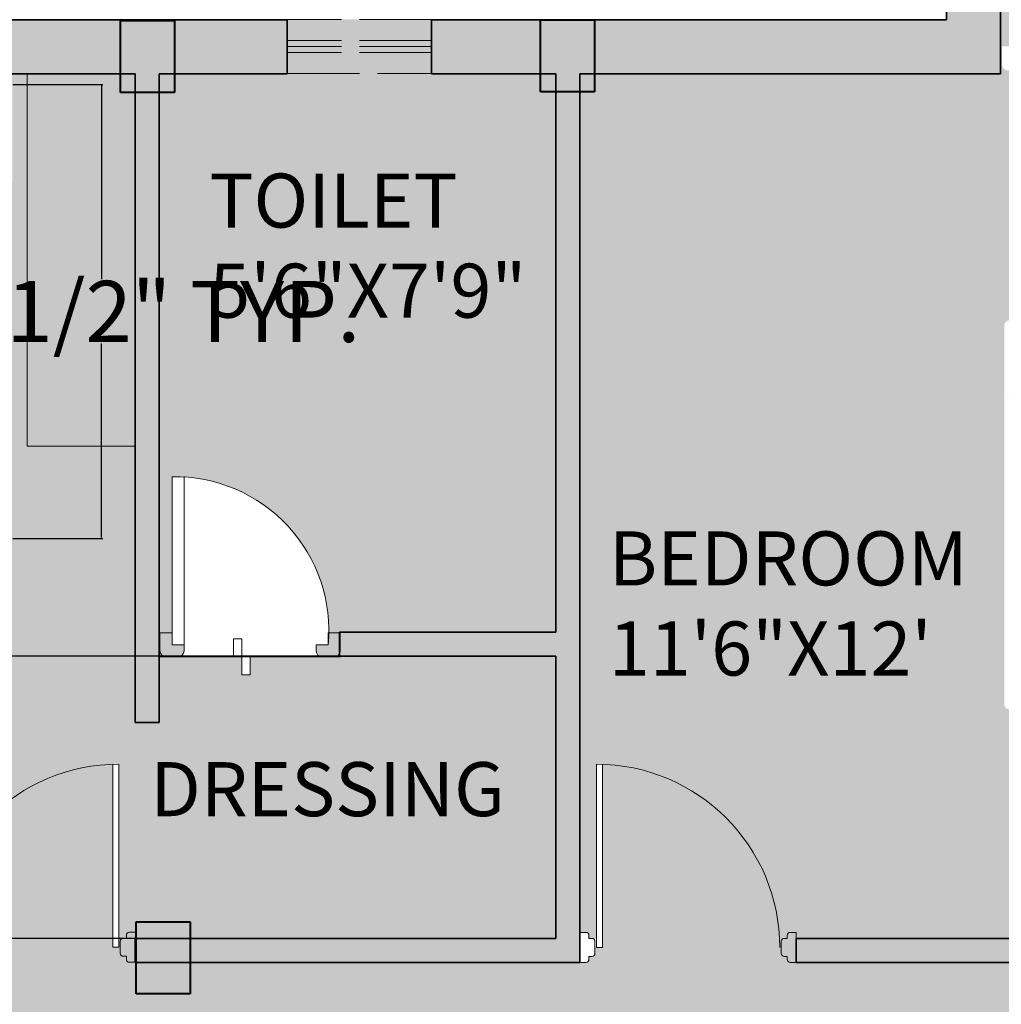
# Model space of a CAD drawing. Units: inches. Extents: x 1077 to 2505, y 1892 to 2728.
# Tile 15 of 26: x 1306 to 1470, y 2422 to 2586. Entities that reach past the tile are written whole.
import ezdxf

# ---------------------------------------------------------------- set-up
doc = ezdxf.new("R2010")
doc.units = ezdxf.units.IN
doc.linetypes.add('ACAD_ISO02W100', pattern=[15, 12, -3])
doc.layers.get('Defpoints').update_dxf_attribs({"color": 220, "linetype": 'ACAD_ISO02W100'})
for name, color, linetype, lineweight in [('00 FURNITURE', 15, 'Continuous', 15), ('A-ANNO-DIMS', 2, 'Continuous', 18), ('A-AREA-IDEN', 7, 'Continuous', 18), ('A-COLS', 7, 'Continuous', 40), ('A-DOOR', 4, 'Continuous', 18), ('A-FLOR-CASE', 8, 'Continuous', 18), ('A-GLAZ-VENT', 6, 'ACAD_ISO02W100', 13), ('A-WALL-PATT', 7, 'Continuous', 9), ('A_FUR 1', 5, 'Continuous', 5), ('WALL', 7, 'Continuous', 35)]:
    doc.layers.add(name, color=color, linetype=linetype, lineweight=lineweight)
doc.layers.add('A-FLOR-CASE-PATT', color=32, linetype='Continuous', lineweight=9, true_color=0xcd6928)
doc.layers.add('A-FLOR-PATT', color=254, linetype='Continuous', lineweight=9, true_color=0xd7ebd2)
doc.styles.get("Standard").update_dxf_attribs({"font": 'arial.ttf'})
doc.dimstyles.get("Standard").update_dxf_attribs({"dimtxt": 10.18, "dimasz": 0.18, "dimexe": 0.18, "dimexo": 0.0625, "dimgap": 0.09, "dimtad": 0, "dimtih": 1, "dimtoh": 1, "dimdec": 0, "dimzin": 0, "dimdsep": 46, "dimlunit": 3, "dimtxsty": 'Standard', "dimcen": 0.09, "dimadec": 0, "dimazin": 0, "dimtfac": 1, "dimtdec": 0, "dimtofl": 0, "dimtmove": 0, "dimatfit": 3, "dimfxl": 1, "dimtolj": 1, "dimtzin": 0, "dimarcsym": 0})

# ---------------------------------------------------------------- blocks, each defined once
blk = doc.blocks.new('DDD')
at = {"layer": '00 FURNITURE'}
for p, q in [((-12579.77, -15859.53), (-12579.77, -15829.05)), ((-12578.77, -15859.53), (-12578.77, -15829.03)), ((-12612.02, -15857.03), (-12612.02, -15862.03)), ((-12611.02, -15857.03), (-12612.02, -15857.03)), ((-12610.52, -15858.03), (-12610.52, -15857.53)), ((-12577.52, -15858.03), (-12577.52, -15857.53)), ((-12577.02, -15857.03), (-12576.02, -15857.03)), ((-12576.02, -15857.03), (-12576.02, -15862.03)), ((-12578.77, -15859.53), (-12579.77, -15859.53)), ((-12610.52, -15861.53), (-12610.52, -15861.03)), ((-12577.52, -15861.53), (-12577.52, -15861.03)), ((-12612.02, -15862.03), (-12611.02, -15862.03)), ((-12576.02, -15862.03), (-12577.02, -15862.03))]:
    blk.add_line(p, q, dxfattribs=at)
for points in [[(-12610.52, -15861.03), (-12610.02, -15861.03, 0.414214), (-12609.52, -15860.53), (-12609.52, -15858.53, 0.414214), (-12610.02, -15858.03), (-12610.52, -15858.03)], [(-12577.52, -15861.03), (-12578.02, -15861.03, -0.414214), (-12578.52, -15860.53), (-12578.52, -15858.53, -0.414214), (-12578.02, -15858.03), (-12577.52, -15858.03)]]:
    blk.add_lwpolyline(points, format="xyb", dxfattribs=at)
for centre, radius, start, end in [((-12578.77, -15859.53), 30.5, 90, 180), ((-12611.02, -15857.53), 0.5, 0, 90), ((-12577.02, -15857.53), 0.5, 90, 180), ((-12611.02, -15861.53), 0.5, 270, 0), ((-12577.02, -15861.53), 0.5, 180, 270)]:
    blk.add_arc(centre, radius, start, end, dxfattribs=at)
blk = doc.blocks.new('ESTSET')
at = {"layer": 'A_FUR 1'}
for p, q in [((-10.44, 4.1), (-10.44, 32.1)), ((-8.44, 4.1), (-8.44, 32.1)), ((-36.44, 6.1), (-36.44, 3.1)), ((-34.44, 6.1), (-36.44, 6.1)), ((-34.44, 4.1), (-34.44, 6.1)), ((-34.44, 4.1), (-34.44, 6.1)), ((-8.44, 4.1), (-8.44, 6.1)), ((-8.44, 6.1), (-6.44, 6.1)), ((-8.44, 4.1), (-8.44, 6.1)), ((-6.44, 6.1), (-6.44, 3.1)), ((-32.44, 4.1), (-34.44, 4.1)), ((-32.44, 4.1), (-34.44, 4.1)), ((-32.44, 3.1), (-32.44, 4.1)), ((-10.44, 3.1), (-10.44, 4.1)), ((-10.44, 4.1), (-8.44, 4.1)), ((-10.44, 4.1), (-8.44, 4.1)), ((-6.44, 2.1), (-36.44, 2.1)), ((-35.44, 2.1), (-33.44, 2.1)), ((-7.44, 2.1), (-9.44, 2.1))]:
    blk.add_line(p, q, dxfattribs=at)
for points in [[(-21.44, 2.1), (-18.67, 2.1), (-18.67, 5.1), (-20.06, 5.1)], [(-20.06, 5.1), (-20.06, -0.91)], [(-21.44, 2.1), (-21.44, -0.91), (-20.06, -0.91)]]:
    blk.add_lwpolyline(points, dxfattribs=at)
for centre, radius, start, end in [((-8.91, 6.46), 25.64, 88.9606, 185.2816), ((-35.44, 3.1), 1, 180, 270), ((-33.44, 3.1), 1, 270, 0), ((-9.44, 3.1), 1, 180, 270), ((-7.44, 3.1), 1, 270, 0)]:
    blk.add_arc(centre, radius, start, end, dxfattribs=at)
blk = doc.blocks.new('C1')
h = blk.add_hatch(color=256)
h.dxf.hatch_style = 1
h.paths.add_polyline_path([(1668.56, 2445.41), (1677.56, 2445.41), (1677.56, 2457.41), (1668.56, 2457.41)])
for p, q in [((1668.56, 2457.41), (1677.56, 2457.41)), ((1668.56, 2445.41), (1668.56, 2457.41)), ((1677.56, 2457.41), (1677.56, 2445.41)), ((1677.56, 2445.41), (1668.56, 2445.41))]:
    blk.add_line(p, q)
blk = doc.blocks.new('VENT-24')
for p, q in [((3.5, 24), (3.5, 0)), ((4.5, 24), (4.5, 0)), ((5.5, 24), (5.5, 0))]:
    blk.add_line(p, q)
blk.add_lwpolyline([(0, 0), (9, 0), (9, 24), (0, 24)], close=True)
blk = doc.blocks.new('*D33')
at = {"layer": 'A-ANNO-DIMS', "color": 0, "lineweight": -2, "transparency": 16777216}
for p, q in [((1305.15, 2575.38), (1320.12, 2575.38)), ((1319.94, 2575.2), (1319.94, 2542.94)), ((1319.94, 2499.96), (1319.94, 2532.23)), ((1305.15, 2499.78), (1320.12, 2499.78))]:
    blk.add_line(p, q, dxfattribs=at)
at = {"layer": 'A-ANNO-DIMS', "color": 0, "transparency": 16777216}
for points in [[(1319.91, 2575.2), (1319.97, 2575.2), (1319.94, 2575.38)], [(1319.91, 2499.96), (1319.97, 2499.96), (1319.94, 2499.78)]]:
    blk.add_solid(points, dxfattribs=at)
at = {"layer": 'Defpoints', "color": 0, "transparency": 16777216}
for p in [(1305.09, 2575.38), (1319.94, 2575.38), (1305.09, 2499.78)]:
    blk.add_point(p, dxfattribs=at)
at = {"layer": 'A-ANNO-DIMS', "color": 0, "transparency": 16777216, "insert": (1319.94, 2537.58), "char_height": 10.18, "attachment_point": 5}
blk.add_mtext('\\A1;6\'-3 1/2" TYP.', dxfattribs=at)
blk = doc.blocks.new('*D64')
at = {"layer": 'A-ANNO-DIMS', "color": 0, "lineweight": -2, "transparency": 16777216}
for p, q in [((1395.47, 2480.16), (1149.43, 2480.16)), ((1149.61, 2479.98), (1149.61, 2461.95)), ((1149.61, 2433.34), (1149.61, 2451.37)), ((1395.47, 2433.16), (1149.43, 2433.16))]:
    blk.add_line(p, q, dxfattribs=at)
at = {"layer": 'A-ANNO-DIMS', "color": 0, "transparency": 16777216}
for points in [[(1149.58, 2479.98), (1149.64, 2479.98), (1149.61, 2480.16)], [(1149.58, 2433.34), (1149.64, 2433.34), (1149.61, 2433.16)]]:
    blk.add_solid(points, dxfattribs=at)
at = {"layer": 'Defpoints', "color": 0, "transparency": 16777216}
for p in [(1149.61, 2480.16), (1395.53, 2480.16), (1395.53, 2433.16)]:
    blk.add_point(p, dxfattribs=at)
at = {"layer": 'A-ANNO-DIMS', "color": 0, "transparency": 16777216, "insert": (1149.61, 2456.66), "char_height": 10.18, "attachment_point": 5}
blk.add_mtext('\\A1;3\'-11"', dxfattribs=at)

msp = doc.modelspace()

# ---------------------------------------------------------------- hatches: boundary and pattern name
at = {"layer": 'A-FLOR-CASE-PATT', "transparency": 33554610}
h = msp.add_hatch(color=256, dxfattribs=at)
h.dxf.hatch_style = 1
h.paths.add_polyline_path([(1325.53, 2577.15), (1307.53, 2577.15), (1307.53, 2515.13), (1325.53, 2515.13)])
h.paths.add_polyline_path([(1476.35, 2451.18), (1476.35, 2433.16), (1547.53, 2433.16), (1547.53, 2437.11), (1547.53, 2451.18)])
at = {"layer": 'A-FLOR-PATT', "transparency": 33554559}
h = msp.add_hatch(color=256, dxfattribs=at)
h.dxf.hatch_style = 1
h.paths.add_polyline_path([(1395.53, 2577.16), (1374.83, 2577.16), (1350.83, 2577.19), (1350.83, 2577.16), (1329.53, 2577.16), (1329.53, 2480.16), (1329.53, 2469.16), (1325.53, 2469.16), (1325.53, 2515.13), (1307.53, 2515.13), (1307.53, 2577.16), (1269.31, 2577.16), (1221.31, 2577.15), (1221.31, 2577.16), (1187.53, 2577.16), (1187.53, 2433.16), (1289.53, 2433.16), (1289.53, 2429.16), (1263.53, 2429.16), (1187.53, 2429.16), (1187.53, 2395.02), (1187.53, 2395.02), (1187.53, 2371.02), (1187.53, 2371.02), (1187.53, 2307.16), (1259.53, 2307.16), (1259.53, 2399.16), (1263.53, 2399.16), (1263.53, 2307.16), (1289.53, 2307.16), (1289.53, 2306.23), (1325.53, 2306.23), (1325.53, 2307.16), (1329.53, 2307.16), (1329.53, 2306.23), (1365.53, 2306.23), (1365.53, 2307.16), (1432.53, 2307.16), (1432.53, 2088.16), (1547.53, 2088.16), (1547.53, 2140.08), (1511.53, 2140.08), (1511.53, 2267.16), (1475.53, 2267.16), (1475.53, 2303.16), (1468.53, 2303.16), (1468.53, 2307.16), (1547.53, 2307.16), (1547.53, 2348.22), (1547.53, 2396.22), (1547.53, 2429.16), (1435.53, 2429.16), (1435.53, 2433.16), (1476.35, 2433.16), (1476.35, 2451.18), (1547.53, 2451.18), (1547.53, 2577.16), (1499.53, 2577.16), (1499.53, 2586.16), (1547.53, 2586.16), (1547.53, 2642.16), (1518.18, 2642.16), (1518.18, 2642.05), (1494.15, 2642.05), (1494.15, 2642.16), (1469.53, 2642.16), (1469.53, 2577.16), (1399.53, 2577.16), (1399.53, 2429.16), (1325.53, 2429.16), (1325.53, 2433.16), (1329.53, 2433.16), (1395.53, 2433.16), (1395.53, 2480.16), (1359.53, 2480.16), (1359.53, 2484.16), (1395.53, 2484.16)])
h.paths.add_polyline_path([(1357.65, 2482.07), (1355.65, 2482.07), (1355.65, 2481.07, 0.414214), (1356.65, 2480.07), (1344.65, 2480.07), (1344.65, 2477.06), (1343.27, 2477.06), (1343.27, 2480.07), (1330.65, 2480.07, -0.414214), (1329.65, 2481.07), (1329.65, 2484.07), (1331.65, 2484.07), (1331.65, 2510.07, -0.446908)], flags=16)
h.paths.add_polyline_path([(1305.09, 2559.18), (1288.89, 2559.18), (1288.89, 2575.38), (1305.09, 2575.38)], flags=16)
h.paths.add_polyline_path([(1304.19, 2560.08), (1289.79, 2560.08), (1289.79, 2574.48), (1304.19, 2574.48)], flags=0)
h.paths.add_polyline_path([(1287.99, 2500.68, -0.414214), (1287.09, 2499.78), (1265.14, 2499.78), (1224.09, 2499.78, -0.414214), (1223.19, 2500.68), (1223.19, 2557.16), (1223.19, 2571.74), (1223.19, 2575.38), (1287.99, 2575.38), (1287.99, 2571.74), (1287.09, 2571.74, -0.414214), (1287.99, 2570.84)], flags=16)
h.paths.add_polyline_path([(1292.98, 2569.05, -1), (1300.92, 2569.05, -1)], flags=0)
h.paths.add_polyline_path([(1293.32, 2569.05, -1), (1300.58, 2569.05, -1)], flags=0)
h.paths.add_polyline_path([(1322.8, 2462.21), (1322.8, 2431.71), (1323.05, 2430.71), (1323.05, 2431.71), (1321.8, 2431.71), (1321.8, 2462.19, 0.404641), (1292.3, 2431.71), (1292.05, 2430.71, -0.414214), (1291.55, 2430.21), (1291.05, 2430.21), (1291.05, 2429.71, -0.414214), (1290.55, 2429.21), (1289.55, 2429.21), (1289.55, 2434.21), (1290.55, 2434.21, -0.414214), (1291.05, 2433.71), (1291.05, 2433.21), (1291.55, 2433.21, -0.414214), (1292.05, 2432.71), (1292.3, 2431.71, -0.414214)], flags=16)
h.paths.add_polyline_path([(1287.82, 2548.28, 0.292232), (1279.17, 2536.8, 0.052719), (1223.93, 2548.28), (1223.28, 2548.28), (1223.28, 2557.16), (1223.93, 2557.16), (1245.42, 2557.16, -0.117785), (1245.77, 2557.93, -0.059418), (1254.87, 2567.02, -0.379859), (1257.28, 2566.88, -0.02509), (1261.41, 2563.32, -0.025935), (1265.65, 2567.02, -0.379859), (1268.06, 2566.88, -0.061767), (1277.52, 2557.43, -0.069393), (1277.82, 2557.16), (1287.82, 2557.16)], flags=0)
h.paths.add_polyline_path([(1263.47, 2548.28), (1260.56, 2548.28, -0.015371), (1258.01, 2546.13, -0.429576), (1255.37, 2546.06, -0.016036), (1252.69, 2548.28), (1223.28, 2548.28), (1223.28, 2554.42), (1246.78, 2554.42, 0.055344), (1255.37, 2546.06, 0.331768), (1257.52, 2545.74, 0.027343), (1262, 2549.64, 0.00919)], flags=0)
h.paths.add_polyline_path([(1295.56, 2568.34), (1296.87, 2569.09), (1296.87, 2570.6, 0.399698), (1295.39, 2569.05, 0.119004)], flags=0)
h.paths.add_polyline_path([(1295.21, 2569.05, -1), (1298.68, 2569.05, -1)], flags=0)
h.paths.add_polyline_path([(1296.95, 2568.96), (1297.03, 2569), (1297.03, 2569.09), (1296.99, 2569.11), (1296.91, 2568.98)], flags=0)
h.paths.add_polyline_path([(1402.28, 2462.19, -0.414214), (1432.78, 2431.69), (1433.03, 2432.69), (1432.78, 2431.69, 0.404641), (1403.28, 2462.17), (1403.28, 2431.69), (1402.03, 2431.69), (1402.03, 2430.69, -0.414214), (1401.53, 2430.19), (1401.03, 2430.19), (1401.03, 2429.69, -0.414214), (1400.53, 2429.19), (1399.53, 2429.19), (1399.53, 2434.19), (1400.53, 2434.19, -0.414214), (1401.03, 2433.69), (1401.03, 2433.19), (1401.53, 2433.19, -0.414214), (1402.03, 2432.69)], flags=16)
h.paths.add_polyline_path([(1470.16, 2535.21, -0.414214), (1471.06, 2536.11), (1527.54, 2536.11), (1542.12, 2536.11), (1545.76, 2536.11), (1545.76, 2471.31), (1542.12, 2471.31), (1542.12, 2472.21, -0.414214), (1541.22, 2471.31), (1471.06, 2471.31, -0.414214), (1470.16, 2472.21), (1470.16, 2494.16)], flags=16)
h.paths.add_polyline_path([(1483.07, 2536.11, 0.253465), (1480.11, 2526.15, 0.2538), (1470.15, 2523.19)], flags=16)
h.paths.add_polyline_path([(1223.19, 2512.69, 0.253465), (1233.14, 2509.74, 0.2538), (1236.1, 2499.77)], flags=16)
h.paths.add_polyline_path([(1469.77, 2578.72), (1469.77, 2581.72), (1471.77, 2581.72), (1471.77, 2607.72, -0.01951), (1473.77, 2607.68), (1473.77, 2579.72), (1473.77, 2578.72, -0.414214), (1472.77, 2577.72), (1470.77, 2577.72, -0.414214)], flags=16)
h.paths.add_polyline_path([(1382.46, 2398.13), (1395.04, 2398.13), (1395.04, 2399.74), (1382.46, 2399.74)], flags=16)
h.paths.add_polyline_path([(1379.94, 2397.18), (1379.94, 2389.82), (1380.5, 2389.82), (1380.5, 2396.05, -0.41429), (1381.06, 2396.61), (1396.47, 2396.61, -0.414213), (1397.03, 2396.05), (1397.03, 2389.82), (1397.59, 2389.82), (1397.59, 2397.18)], flags=16)
h.paths.add_polyline_path([(1263.37, 2428.14), (1263.37, 2426.14, -0.414214), (1262.37, 2425.14), (1261.37, 2425.14), (1233.41, 2425.14, 0.400854), (1259.37, 2401.04), (1259.37, 2401.14), (1261.37, 2401.14, -0.446908), (1233.37, 2427.14), (1259.37, 2427.14), (1259.37, 2429.14), (1262.37, 2429.14, -0.414214)], flags=16)
h.paths.add_polyline_path([(1404.79, 2398.13), (1417.37, 2398.13), (1417.37, 2399.74), (1404.79, 2399.74)], flags=16)
h.paths.add_polyline_path([(1402.27, 2397.18), (1404.79, 2398.13), (1417.37, 2398.13), (1419.92, 2397.18)], flags=16)
h.paths.add_polyline_path([(1432.26, 2383.16), (1432.26, 2370.59), (1433.87, 2370.59), (1433.87, 2383.16)], flags=16)
h.paths.add_polyline_path([(1431.3, 2385.69), (1423.84, 2385.69), (1423.84, 2385.13), (1430.18, 2385.13, -0.41429), (1430.74, 2384.57), (1430.74, 2369.16, -0.414237), (1430.18, 2368.6), (1423.84, 2368.6), (1423.84, 2368.03), (1431.3, 2368.03)], flags=16)
h.paths.add_polyline_path([(1417.37, 2351.16), (1417.37, 2349.54), (1418.9, 2349.54, 0.414236), (1419.92, 2350.56), (1419.92, 2352.11)], flags=16)
h.paths.add_polyline_path([(1395.04, 2351.16), (1395.04, 2349.54), (1396.58, 2349.54, 0.414235), (1397.59, 2350.56), (1397.59, 2352.11)], flags=16)
h.paths.add_polyline_path([(1366.7, 2370.05), (1365.09, 2370.05), (1365.09, 2368.52, 0.414235), (1366.11, 2367.5), (1367.66, 2367.5)], flags=16)
h.paths.add_polyline_path([(1419.36, 2359.47), (1419.36, 2353.24, -0.41419), (1418.8, 2352.68), (1403.39, 2352.68, -0.414137), (1402.83, 2353.24), (1402.83, 2359.47), (1397.03, 2359.47), (1397.03, 2353.24, -0.414189), (1396.47, 2352.68), (1381.06, 2352.68, -0.414137), (1380.5, 2353.24), (1380.5, 2359.47)], flags=16)
h.paths.add_polyline_path([(1222.29, 2559.18), (1206.09, 2559.18), (1206.09, 2575.38), (1222.29, 2575.38)], flags=16)
h.paths.add_polyline_path([(1221.39, 2560.08), (1206.99, 2560.08), (1206.99, 2574.48), (1221.39, 2574.48)], flags=0)
h.paths.add_polyline_path([(1482, 2577.72), (1482, 2580.73), (1483.38, 2580.73), (1483.38, 2577.72), (1484.77, 2577.72), (1484.77, 2574.72), (1483.38, 2574.72), (1483.38, 2577.72)], flags=16)
h.paths.add_polyline_path([(1266.37, 2415.53), (1266.37, 2414.14), (1263.37, 2414.14), (1263.37, 2415.53), (1260.36, 2415.53), (1260.36, 2416.91), (1263.37, 2416.91), (1263.37, 2415.53)], flags=16)
h.paths.add_polyline_path([(1210.26, 2569.05, -1), (1218.19, 2569.05, -1)], flags=0)
h.paths.add_polyline_path([(1210.6, 2569.05, -1), (1217.85, 2569.05, -1)], flags=0)
h.paths.add_polyline_path([(1212.84, 2568.34), (1214.15, 2569.09), (1214.15, 2570.6, 0.399698), (1212.67, 2569.05, 0.119004)], flags=0)
h.paths.add_polyline_path([(1212.49, 2569.05, -1), (1215.96, 2569.05, -1)], flags=0)
h.paths.add_polyline_path([(1214.23, 2568.96), (1214.3, 2568.91), (1214.3, 2569)], flags=0)
h.paths.add_polyline_path([(1507.18, 2480.12, 0.052719), (1518.66, 2535.36), (1518.66, 2536.01), (1527.54, 2536.01), (1527.54, 2535.36), (1527.54, 2513.88, -0.117785), (1528.31, 2513.53, -0.059418), (1537.4, 2504.43, -0.379859), (1537.26, 2502.01, -0.02509), (1533.7, 2497.89, -0.025935), (1537.4, 2493.64, -0.379859), (1537.26, 2491.23, -0.061767), (1527.8, 2481.77, -0.069393), (1527.54, 2481.47), (1527.54, 2471.47), (1518.66, 2471.47, 0.292232)], flags=0)
h.paths.add_polyline_path([(1516.43, 2503.92, -0.016036), (1518.66, 2506.6), (1518.66, 2536.01), (1524.8, 2536.01), (1524.8, 2512.51, 0.055344), (1516.43, 2503.92, 0.331768), (1516.12, 2501.77, 0.027343), (1520.01, 2497.29, 0.00919), (1518.66, 2495.82), (1518.66, 2498.73, -0.015371), (1516.5, 2501.28, -0.429576)], flags=0)
h.paths.add_polyline_path([(1499.63, 2625.5, -0.171636), (1502.82, 2631.01), (1502.82, 2633.37), (1498.68, 2633.37, -0.414214), (1497.7, 2634.36), (1497.7, 2640.66, -0.414214), (1498.68, 2641.64), (1514.82, 2641.64, -0.414214), (1515.81, 2640.66), (1515.81, 2634.36, -0.414214), (1514.82, 2633.37), (1510.69, 2633.37), (1510.69, 2631.01, -0.171636), (1513.88, 2625.5, -0.258205), (1509.31, 2614.47), (1504.19, 2614.47, -0.258205)], flags=16)
h.paths.add_polyline_path([(1501.2, 2625.5, -0.171636), (1504.39, 2631.01), (1509.12, 2631.01, -0.171636), (1512.3, 2625.5, -0.210384), (1509.35, 2616.02), (1504.16, 2616.02, -0.210384)], flags=0)
h.paths.add_polyline_path([(1529.56, 2537.01), (1529.56, 2553.21), (1545.76, 2553.21), (1545.76, 2537.01)], flags=16)
h.paths.add_polyline_path([(1530.46, 2537.91), (1530.46, 2552.31), (1544.86, 2552.31), (1544.86, 2537.91)], flags=0)
h.paths.add_polyline_path([(1535.45, 2545.07, -1), (1543.39, 2545.07, -1)], flags=0)
h.paths.add_polyline_path([(1535.8, 2545.07, -1), (1543.05, 2545.07, -1)], flags=0)
h.paths.add_polyline_path([(1529.56, 2470.41), (1545.76, 2470.41), (1545.76, 2454.21), (1529.56, 2454.21)], flags=16)
h.paths.add_polyline_path([(1541.16, 2544.99), (1540.98, 2544.99, -0.544606), (1538.71, 2543.68), (1538.62, 2543.53, 0.547962)], flags=0)
h.paths.add_polyline_path([(1530.46, 2469.51), (1544.86, 2469.51), (1544.86, 2455.11), (1530.46, 2455.11)], flags=0)
h.paths.add_polyline_path([(1539.47, 2545.14), (1539.42, 2545.22), (1539.38, 2545.14)], flags=0)
h.paths.add_polyline_path([(1543.39, 2462.34, -1), (1535.45, 2462.34, -1)], flags=0)
h.paths.add_polyline_path([(1543.05, 2462.34, -1), (1535.8, 2462.34, -1)], flags=0)
h.paths.add_polyline_path([(1541.16, 2462.27), (1540.98, 2462.27, -0.544606), (1538.71, 2460.96), (1538.62, 2460.8, 0.547962)], flags=0)
h.paths.add_polyline_path([(1539.47, 2462.42), (1539.42, 2462.5), (1539.38, 2462.42)], flags=0)
h.paths.add_polyline_path([(1435.32, 2335.25, -0.414214), (1465.82, 2304.75), (1466.07, 2305.75), (1465.82, 2304.75, 0.404641), (1436.32, 2335.23), (1436.32, 2304.75), (1435.07, 2304.75), (1435.07, 2303.75, -0.414214), (1434.57, 2303.25), (1434.07, 2303.25), (1434.07, 2302.75, -0.414214), (1433.57, 2302.25), (1432.57, 2302.25), (1432.57, 2307.25), (1433.57, 2307.25, -0.414214), (1434.07, 2306.75), (1434.07, 2306.25), (1434.57, 2306.25, -0.414214), (1435.07, 2305.75)], flags=16)
h.paths.add_polyline_path([(1532.13, 2635.71), (1535.43, 2635.71), (1535.43, 2635.89), (1532.13, 2635.89)], flags=16)
edge = h.paths.add_edge_path(flags=16)
edge.add_arc((1535.98, 2632.67), 0.183, 270, 360)
edge.add_line((1536.17, 2632.67), (1536.17, 2639.82))
edge.add_line((1536.17, 2639.82), (1538.29, 2639.82))
edge.add_line((1538.29, 2639.82), (1538.29, 2641.82))
edge.add_line((1538.29, 2641.82), (1533.25, 2641.82))
edge.add_line((1533.25, 2641.82), (1533.25, 2639.82))
edge.add_line((1533.25, 2639.82), (1534.87, 2639.82))
edge.add_line((1534.87, 2639.82), (1534.87, 2639))
edge.add_line((1534.87, 2639), (1533.7, 2639))
edge.add_line((1533.7, 2639), (1533.7, 2639.82))
edge.add_line((1533.7, 2639.82), (1533.25, 2639.82))
edge.add_line((1533.25, 2639.82), (1533.25, 2641.82))
edge.add_line((1533.25, 2641.82), (1538.29, 2641.82))
edge.add_line((1538.29, 2641.82), (1538.29, 2641.34))
edge.add_line((1538.29, 2641.34), (1540.64, 2641.58))
edge.add_line((1540.64, 2641.58), (1540.64, 2641.82))
edge.add_line((1540.64, 2641.82), (1541.5, 2641.82))
edge.add_line((1541.5, 2641.82), (1541.5, 2641.25))
edge.add_line((1541.5, 2641.25), (1541.31, 2639.79))
edge.add_ellipse((1541.09, 2638.95), major_axis=(-1.08, 0), ratio=0.790849, start_angle=180, end_angle=255.2976, ccw=False)
edge.add_line((1542.17, 2638.95), (1542.17, 2638.38))
edge.add_ellipse((1541.09, 2638.38), major_axis=(-1.08, 0), ratio=0.790849, start_angle=0, end_angle=180, ccw=False)
edge.add_line((1540, 2638.38), (1540.01, 2638.87))
edge.add_ellipse((1541.09, 2638.95), major_axis=(-1.08, 0), ratio=0.790849, start_angle=284.7024, end_angle=364.0401, ccw=False)
edge.add_line((1540.78, 2639.75), (1540.78, 2641.25))
edge.add_line((1540.78, 2641.25), (1540.64, 2641.25))
edge.add_line((1540.64, 2641.25), (1538.29, 2641.01))
edge.add_line((1538.29, 2641.01), (1538.29, 2639.82))
edge.add_line((1538.29, 2639.82), (1536.17, 2639.82))
edge.add_line((1536.17, 2639.82), (1536.17, 2632.48))
edge.add_line((1536.17, 2632.48), (1535.98, 2632.48))
h.paths.add_polyline_path([(1496.32, 2250.34, -0.292371), (1498.9, 2247.83, -0.085148), (1501.21, 2208.85, -0.01331), (1500.27, 2098.5, -0.379287), (1497.22, 2095.28, -0.0502), (1441.54, 2095.28, -0.379287), (1438.5, 2098.5, -0.01331), (1437.56, 2208.85, -0.086132), (1439.96, 2248.26, -0.295116), (1442.59, 2250.78, -0.114238)], flags=16)
h.paths.add_polyline_path([(1495.16, 2205.84, -0.355389), (1496.7, 2202.1), (1492.94, 2189.65, -0.398275), (1489.12, 2187.47, 0.113332), (1449.64, 2187.47, -0.398275), (1445.82, 2189.65), (1442.06, 2202.1, -0.355394), (1443.6, 2205.84, -0.265725)], flags=0)
h.paths.add_polyline_path([(1440.37, 2195.72), (1445.94, 2181.67), (1445.94, 2160.63), (1440.84, 2157.26)], flags=0)
h.paths.add_polyline_path([(1498.46, 2195.72), (1497.99, 2157.26), (1492.88, 2160.63), (1492.88, 2181.67)], flags=0)
h.paths.add_polyline_path([(1445.94, 2158.37), (1445.94, 2137.12), (1441.12, 2122.56), (1440.87, 2155.03)], flags=0)
h.paths.add_polyline_path([(1492.88, 2158.37), (1497.96, 2155.03), (1497.71, 2122.56), (1492.88, 2137.12)], flags=0)
h.paths.add_polyline_path([(1489.88, 2130.4), (1494.39, 2107.67, -0.090102), (1444.44, 2107.65), (1448.95, 2130.39, 0.036636)], flags=0)
h.paths.add_polyline_path([(1447.54, 2159.34), (1497.44, 2159.34), (1497.44, 2177.89), (1447.54, 2177.89)], flags=8)
h.paths.add_polyline_path([(1196.44, 2354.84), (1246.65, 2354.84), (1246.65, 2388.43), (1196.44, 2388.43)], flags=24)
h.paths.add_polyline_path([(1296.09, 2360.25), (1353.81, 2360.25), (1353.81, 2393.84), (1296.09, 2393.84)], flags=24)
h.paths.add_polyline_path([(1400.72, 2471.85), (1470.63, 2471.85), (1470.63, 2505.44), (1400.72, 2505.44)], flags=24)
h.paths.add_polyline_path([(1324.78, 2448.48), (1394.95, 2448.48), (1394.95, 2467.02), (1324.78, 2467.02)], flags=24)
h.paths.add_polyline_path([(1335.08, 2531.43), (1389.67, 2531.43), (1389.67, 2565.02), (1335.08, 2565.02)], flags=24)
h.paths.add_polyline_path([(1225.76, 2460), (1295.67, 2460), (1295.67, 2493.58), (1225.76, 2493.58)], flags=24)
h = msp.add_hatch(color=256, dxfattribs=at)
h.dxf.hatch_style = 1
h.paths.add_polyline_path([(1547.53, 2348.22), (1547.53, 2396.22), (1547.53, 2425.11), (1547.53, 2425.11), (1547.53, 2429.16), (1435.53, 2429.16), (1434.03, 2429.21), (1434.03, 2430.19), (1433.03, 2430.19), (1432.78, 2431.69, 0.404641), (1403.28, 2462.17), (1403.28, 2431.69), (1402.03, 2431.69), (1402.03, 2430.19), (1401.03, 2430.19), (1401.03, 2429.19), (1399.53, 2429.19), (1399.53, 2429.19), (1399.53, 2429.16), (1334.67, 2429.16), (1334.67, 2423.95), (1325.67, 2423.95), (1325.67, 2429.16), (1325.53, 2429.16), (1324.05, 2429.24), (1324.05, 2430.21), (1323.05, 2430.21), (1323.05, 2431.71), (1321.8, 2431.71), (1321.8, 2462.19, 0.416544), (1292.05, 2430.73, -0.423614), (1291.55, 2430.21), (1291.05, 2430.21), (1291.05, 2429.21), (1289.55, 2429.21), (1289.53, 2429.21), (1289.53, 2429.16), (1263.37, 2429.16), (1263.37, 2415.53), (1266.37, 2415.53), (1266.37, 2414.14), (1263.37, 2414.14), (1263.37, 2399.16), (1263.53, 2399.16), (1263.53, 2307.16), (1289.53, 2307.16), (1289.53, 2306.23), (1323.26, 2306.23), (1323.26, 2307.21), (1332.26, 2307.21), (1365.53, 2306.23), (1365.53, 2307.16), (1432.53, 2307.16), (1432.57, 2307.16), (1432.57, 2307.25), (1434.07, 2307.25), (1434.07, 2306.25), (1435.32, 2306.25), (1435.32, 2335.25, -0.407346), (1466.07, 2305.73, -0.423614), (1466.57, 2306.25), (1467.07, 2306.25), (1467.07, 2307.25), (1468.57, 2307.25), (1547.53, 2307.16), (1547.53, 2307.2)])
h.paths.add_polyline_path([(1430.74, 2369.16), (1430.74, 2384.57, 0.41429), (1430.18, 2385.13), (1423.84, 2385.13), (1423.84, 2368.6), (1430.18, 2368.6, 0.414237)], flags=16)
h.paths.add_polyline_path([(1432.26, 2383.16), (1432.26, 2370.59), (1433.87, 2370.59), (1433.87, 2383.16)], flags=16)
h.paths.add_polyline_path([(1431.3, 2368.03), (1431.3, 2385.69), (1432.26, 2383.16), (1432.26, 2370.59)], flags=16)
h.paths.add_polyline_path([(1417.37, 2351.16), (1417.37, 2349.54), (1418.9, 2349.54, 0.414236), (1419.92, 2350.56), (1419.92, 2352.11)], flags=16)
h.paths.add_polyline_path([(1403.39, 2352.68), (1418.78, 2352.68, 0.42427), (1419.36, 2353.24), (1419.36, 2359.47), (1402.83, 2359.47), (1402.83, 2353.24, 0.414137)], flags=16)
h.paths.add_polyline_path([(1366.7, 2370.05), (1365.09, 2370.05), (1365.09, 2368.52, 0.414235), (1366.11, 2367.5), (1367.66, 2367.5)], flags=16)
h.paths.add_polyline_path([(1382.46, 2398.13), (1395.04, 2398.13), (1395.04, 2399.74), (1382.46, 2399.74)], flags=16)
h.paths.add_polyline_path([(1396.47, 2396.61), (1381.06, 2396.61, 0.41429), (1380.5, 2396.05), (1380.5, 2389.82), (1397.03, 2389.82), (1397.03, 2396.05, 0.414213)], flags=16)
h.paths.add_polyline_path([(1402.27, 2397.18), (1402.83, 2396.05, -0.414213), (1403.39, 2396.61)], flags=16)
h.paths.add_polyline_path([(1418.8, 2396.61), (1419.36, 2396.61), (1419.36, 2396.05, 0.414237)], flags=16)
h.paths.add_polyline_path([(1404.79, 2398.13), (1417.37, 2398.13), (1417.37, 2399.74), (1404.79, 2399.74)], flags=16)
h.paths.add_polyline_path([(1381.06, 2352.68, -0.414213), (1380.5, 2353.24), (1380.27, 2352.11)], flags=16)
h.paths.add_polyline_path([(1396.58, 2349.54), (1396.58, 2349.54), (1395.04, 2349.54), (1395.04, 2349.54), (1382.46, 2349.54), (1382.46, 2351.16), (1395.04, 2351.16), (1397.59, 2352.11), (1397.59, 2350.56, -0.414235)], flags=16)
h.paths.add_polyline_path([(1379.94, 2397.18), (1382.46, 2398.13), (1395.04, 2398.13), (1397.59, 2397.18)], flags=16)
h.paths.add_polyline_path([(1368.78, 2384.59, 0.414213), (1368.22, 2384.03), (1367.66, 2367.5), (1367.66, 2385.15)], flags=16)
h.paths.add_polyline_path([(1547.53, 2574.38), (1547.51, 2574.38), (1547.51, 2577.16), (1499.53, 2577.16), (1484.77, 2577.44), (1484.77, 2574.72), (1483.38, 2574.72), (1483.38, 2577.72), (1482, 2577.72), (1469.53, 2577.72), (1469.53, 2577.16), (1401.95, 2577.16), (1401.95, 2574.12), (1399.53, 2574.12), (1399.53, 2434.19), (1401.03, 2434.19), (1401.03, 2433.19), (1402.28, 2433.19), (1402.28, 2462.19, -0.407346), (1433.03, 2432.67, -0.423614), (1433.53, 2433.19), (1434.03, 2433.19), (1434.03, 2434.19), (1435.53, 2434.19), (1476.35, 2433.81), (1476.35, 2451.18), (1547.53, 2451.18)])
h.paths.add_polyline_path([(1470.16, 2535.21, -0.414214), (1471.06, 2536.11), (1527.54, 2536.11), (1542.12, 2536.11), (1545.76, 2536.11), (1545.76, 2471.31), (1542.12, 2471.31), (1542.12, 2472.21, -0.414214), (1541.22, 2471.31), (1471.06, 2471.31, -0.414214), (1470.16, 2472.21), (1470.16, 2494.16)], flags=16)
h.paths.add_polyline_path([(1483.07, 2536.11, 0.253465), (1480.11, 2526.15, 0.2538), (1470.15, 2523.19)], flags=16)
h.paths.add_polyline_path([(1525.55, 2481.52, -0.000893), (1524.8, 2482.24), (1524.8, 2471.47), (1527.54, 2471.47), (1527.54, 2472.12), (1527.54, 2481.47, -0.388819)], flags=0)
h.paths.add_polyline_path([(1518.66, 2536.01), (1527.54, 2536.01), (1527.54, 2535.36), (1527.54, 2513.88, -0.117785), (1528.31, 2513.53, -0.059418), (1537.4, 2504.43, -0.379859), (1537.26, 2502.01, -0.02509), (1533.7, 2497.89, 0.033431), (1528.3, 2502.74, 0.308459), (1526.25, 2502.88, 0.047827), (1518.66, 2495.82), (1518.66, 2498.73, -0.015371), (1516.5, 2501.28, -0.429576), (1516.43, 2503.92, -0.016036), (1518.66, 2506.6)], flags=0)
h.paths.add_polyline_path([(1529.56, 2537.01), (1529.56, 2553.21), (1545.76, 2553.21), (1545.76, 2537.01)], flags=16)
h.paths.add_polyline_path([(1530.46, 2537.91), (1530.46, 2552.31), (1544.86, 2552.31), (1544.86, 2537.91)], flags=0)
h.paths.add_polyline_path([(1535.8, 2545.07, -1), (1543.05, 2545.07, -1)], flags=0)
h.paths.add_polyline_path([(1541.16, 2544.99), (1540.98, 2544.99, -0.544606), (1538.71, 2543.68), (1538.62, 2543.53, 0.547962)], flags=0)
h.paths.add_polyline_path([(1539.47, 2545.14), (1539.42, 2545.22), (1539.38, 2545.14)], flags=0)
h.paths.add_polyline_path([(1529.56, 2470.41), (1545.76, 2470.41), (1545.76, 2454.21), (1529.56, 2454.21)], flags=16)
h.paths.add_polyline_path([(1530.46, 2469.51), (1544.86, 2469.51), (1544.86, 2455.11), (1530.46, 2455.11)], flags=0)
h.paths.add_polyline_path([(1535.8, 2462.34, -1), (1543.05, 2462.34, -1)], flags=0)
h.paths.add_polyline_path([(1541.16, 2462.27), (1540.98, 2462.27, -0.544606), (1538.71, 2460.96), (1538.62, 2460.8, 0.547962)], flags=0)
h.paths.add_polyline_path([(1539.47, 2462.42), (1539.42, 2462.5), (1539.38, 2462.42)], flags=0)
h.paths.add_polyline_path([(1395.53, 2574.12), (1392.95, 2574.12), (1392.95, 2577.16), (1374.83, 2577.16), (1350.83, 2577.19), (1350.83, 2577.16), (1332.07, 2577.16), (1332.07, 2574), (1329.53, 2574), (1329.53, 2484.07), (1331.65, 2484.07), (1331.65, 2510.07, -0.423677), (1357.76, 2484.07), (1359.53, 2484.07), (1359.53, 2484.16), (1395.53, 2484.16)], flags=17)
h.paths.add_polyline_path([(1395.53, 2480.16), (1359.06, 2480.16, 0.437533), (1359.53, 2481.55), (1359.53, 2484.16), (1395.53, 2484.16), (1395.53, 2574.12), (1392.95, 2574.12), (1392.95, 2577.16), (1374.83, 2577.16), (1350.83, 2577.19), (1350.83, 2577.16), (1332.07, 2577.16), (1332.07, 2574), (1329.53, 2574), (1329.53, 2484.07), (1329.65, 2484.07), (1329.65, 2481.07), (1329.53, 2480.16), (1329.53, 2469.16), (1325.53, 2469.16), (1325.53, 2515.13), (1307.53, 2515.13), (1307.53, 2577.16), (1269.31, 2577.16), (1221.31, 2577.15), (1221.31, 2577.16), (1187.61, 2577.16), (1187.61, 2574.03), (1187.53, 2433.16), (1289.55, 2433.16), (1289.55, 2434.21), (1291.05, 2434.21), (1291.05, 2433.21), (1292.05, 2433.21), (1292.3, 2431.71, -0.414214), (1322.8, 2462.21), (1323.05, 2432.71, -0.414214), (1323.55, 2433.21), (1324.05, 2433.21), (1324.05, 2434.21), (1325.67, 2434.21), (1325.67, 2435.95), (1334.67, 2435.95), (1334.67, 2433.16), (1395.53, 2433.16)])
h.paths.add_polyline_path([(1344.65, 2480.07), (1344.65, 2477.06), (1343.27, 2477.06), (1343.27, 2480.07), (1332.65, 2480.07, 0.414214), (1333.65, 2481.07), (1333.65, 2482.07), (1331.65, 2482.07), (1331.65, 2484.07), (1331.65, 2510.07, -0.446908), (1357.65, 2482.07), (1355.65, 2482.07), (1355.65, 2481.07, 0.414214), (1356.65, 2480.07)], flags=16)
h.paths.add_polyline_path([(1287.99, 2500.68, -0.414214), (1287.09, 2499.78), (1265.14, 2499.78), (1224.09, 2499.78, -0.414214), (1223.19, 2500.68), (1223.19, 2557.16), (1223.19, 2571.74), (1223.19, 2575.38), (1287.99, 2575.38), (1287.99, 2571.74), (1287.09, 2571.74, -0.414214), (1287.99, 2570.84)], flags=16)
h.paths.add_polyline_path([(1277.77, 2555.17, -0.000893), (1277.05, 2554.42), (1287.82, 2554.42), (1287.82, 2557.16), (1287.17, 2557.16), (1277.82, 2557.16, -0.388819)], flags=0)
h.paths.add_polyline_path([(1223.28, 2548.28), (1223.28, 2557.16), (1223.93, 2557.16), (1245.42, 2557.16, -0.117785), (1245.77, 2557.93, -0.059418), (1254.87, 2567.02, -0.379859), (1257.28, 2566.88, -0.02509), (1261.41, 2563.32, 0.033431), (1256.55, 2557.93, 0.308459), (1256.41, 2555.88, 0.047827), (1263.47, 2548.28), (1260.56, 2548.28, -0.015371), (1258.01, 2546.13, -0.429576), (1255.37, 2546.06, -0.016036), (1252.69, 2548.28)], flags=0)
h.paths.add_polyline_path([(1305.09, 2559.18), (1288.89, 2559.18), (1288.89, 2575.38), (1305.09, 2575.38)], flags=16)
h.paths.add_polyline_path([(1304.19, 2560.08), (1289.79, 2560.08), (1289.79, 2574.48), (1304.19, 2574.48)], flags=0)
h.paths.add_polyline_path([(1300.58, 2569.05, -1), (1293.32, 2569.05, -1)], flags=0)
h.paths.add_polyline_path([(1223.19, 2512.69, 0.253465), (1233.14, 2509.74, 0.2538), (1236.1, 2499.77)], flags=16)
h.paths.add_polyline_path([(1295.56, 2568.34), (1296.87, 2569.09), (1296.87, 2570.6, 0.399698), (1295.39, 2569.05, 0.119004)], flags=0)
h.paths.add_polyline_path([(1295.21, 2569.05, -1), (1298.68, 2569.05, -1)], flags=0)
h.paths.add_polyline_path([(1296.95, 2568.96), (1297.03, 2569), (1297.03, 2569.09), (1296.99, 2569.11), (1296.91, 2568.98)], flags=0)
h.paths.add_polyline_path([(1222.29, 2559.18), (1206.09, 2559.18), (1206.09, 2575.38), (1222.29, 2575.38)], flags=16)
h.paths.add_polyline_path([(1221.39, 2560.08), (1206.99, 2560.08), (1206.99, 2574.48), (1221.39, 2574.48)], flags=0)
h.paths.add_polyline_path([(1217.85, 2569.05, -1), (1210.6, 2569.05, -1)], flags=0)
h.paths.add_polyline_path([(1212.84, 2568.34), (1214.15, 2569.09), (1214.15, 2570.6, 0.399698), (1212.67, 2569.05, 0.119004)], flags=0)
h.paths.add_polyline_path([(1212.49, 2569.05, -1), (1215.96, 2569.05, -1)], flags=0)
h.paths.add_polyline_path([(1214.23, 2568.96), (1214.3, 2569), (1214.3, 2569.09), (1214.26, 2569.11), (1214.19, 2568.98)], flags=0)
h.paths.add_polyline_path([(1259.53, 2399.14), (1259.37, 2399.14), (1259.37, 2401.04, -0.423677), (1233.37, 2427.14), (1259.37, 2427.14), (1259.37, 2429.16), (1187.53, 2429.16), (1187.53, 2395.02), (1187.53, 2395.02), (1187.53, 2371.02), (1187.53, 2371.02), (1187.53, 2311.49), (1187.55, 2311.49), (1187.55, 2307.16), (1259.53, 2307.16)])
h.paths.add_polyline_path([(1323.26, 2295.21), (1323.26, 2304.23), (1289.53, 2304.23), (1289.53, 2303.16), (1187.55, 2303.16), (1187.55, 2299.49), (1178.53, 2299.49), (1178.53, 2267.66), (1178.53, 2219.66), (1182.03, 2219.66), (1182.03, 2267.67), (1184.03, 2267.67), (1184.03, 2219.66), (1187.53, 2219.66), (1187.53, 2153.16), (1228.13, 2153.16), (1276.13, 2153.16), (1276.13, 2153.16), (1324.54, 2153.16), (1324.54, 2154.67), (1325.54, 2154.67), (1325.54, 2155.92), (1296.54, 2155.92, -0.407346), (1326.06, 2186.67, -0.423614), (1325.54, 2187.17), (1325.54, 2187.67), (1324.54, 2187.67), (1324.54, 2189.17), (1325.43, 2295.21)])
h.paths.add_polyline_path([(1432.53, 2307.16), (1365.53, 2307.16), (1365.53, 2306.23), (1365.53, 2303.16), (1428.53, 2303.16), (1428.53, 2221.2), (1428.57, 2221.2), (1428.57, 2197.2), (1428.53, 2197.16), (1428.53, 2303.01), (1404.46, 2303.01), (1404.46, 2221.2), (1329.53, 2221.2), (1329.53, 2307.16), (1325.53, 2307.16), (1325.53, 2295.21), (1325.43, 2295.21), (1324.54, 2189.17), (1324.54, 2187.67), (1326.04, 2187.67, 1.016365), (1326.06, 2186.67, 0.407348), (1296.54, 2155.92), (1325.54, 2155.92), (1325.54, 2154.67), (1324.54, 2154.67), (1324.54, 2153.16), (1329.53, 2153.16), (1329.53, 2144.16), (1432.53, 2144.16)])
h.paths.add_polyline_path([(1361.95, 2194.26), (1361.95, 2193.16), (1329.53, 2193.16), (1329.53, 2189.16), (1329.54, 2188.17), (1329.54, 2189.16), (1329.53, 2189.16), (1329.53, 2193.16), (1361.95, 2193.16), (1361.95, 2196.26), (1409.95, 2196.26), (1409.95, 2194.26)], flags=16)
h.paths.add_polyline_path([(1377.02, 2200.5), (1345.91, 2200.5), (1345.91, 2218.4), (1347.87, 2218.4), (1347.87, 2219.18), (1374.75, 2219.18), (1374.75, 2218.4), (1377.02, 2218.4)], flags=16)
h.paths.add_polyline_path([(1367.07, 2210.7, -1), (1373.34, 2210.7, -1)], flags=0)
h.paths.add_polyline_path([(1349.92, 2210.7, -1), (1356.98, 2210.7, -1)], flags=0)
h.paths.add_polyline_path([(1405.95, 2256.57), (1405.95, 2277.6), (1427.86, 2277.6), (1427.86, 2256.57)], flags=16)
h.paths.add_polyline_path([(1412.92, 2258.68, -0.414201), (1410.93, 2260.67), (1410.93, 2273.62, -0.414239), (1412.92, 2275.61), (1423.88, 2275.61, -0.414227), (1425.87, 2273.62), (1425.87, 2260.67, -0.414214), (1423.88, 2258.68)], flags=0)
h.paths.add_polyline_path([(1407.61, 2263.66, -1), (1409.18, 2263.66, -1)], flags=0)
h.paths.add_polyline_path([(1407.61, 2267.14, -1), (1409.18, 2267.14, -1)], flags=0)
h.paths.add_polyline_path([(1416.91, 2267.15, -1), (1419.89, 2267.15, -1)], flags=0)
h.paths.add_polyline_path([(1407.61, 2270.63, -1), (1409.18, 2270.63, -1)], flags=0)
h.paths.add_polyline_path([(1475.53, 2303.16), (1468.57, 2303.16), (1468.57, 2302.25), (1467.07, 2302.25), (1467.07, 2303.25), (1466.07, 2303.25), (1465.82, 2304.75, 0.404641), (1436.32, 2335.23), (1436.32, 2304.75), (1435.07, 2304.75), (1435.07, 2303.25), (1434.07, 2303.25), (1434.07, 2302.25), (1432.53, 2302.25), (1432.53, 2144.16), (1432.53, 2088.16), (1547.52, 2088.16), (1547.52, 2100.19), (1547.52, 2140.08), (1511.53, 2140.08), (1511.53, 2267.16), (1475.53, 2267.16)])
h.paths.add_polyline_path([(1438.35, 2102.86, 0.033498), (1438.37, 2102.21, -0.000079)], flags=16)
h.paths.add_polyline_path([(1496.32, 2250.34, -0.292371), (1498.9, 2247.83, -0.085148), (1501.21, 2208.85, -0.012784), (1500.42, 2102.86, -0.033498), (1500.39, 2102.21, 0.012863), (1501.21, 2208.85, 0.077283), (1499.67, 2244.3, 0.265882), (1497.48, 2246.8, 0.14401), (1441.46, 2247.36, 0.270646), (1439.21, 2244.85, -0.007564), (1439.96, 2248.26, -0.295116), (1442.59, 2250.78, -0.114238)], flags=16)
h.paths.add_polyline_path([(1495.16, 2205.84, -0.355389), (1496.7, 2202.1), (1492.94, 2189.65, -0.398275), (1489.12, 2187.47, 0.113332), (1449.64, 2187.47, -0.398275), (1445.82, 2189.65), (1442.06, 2202.1, -0.355394), (1443.6, 2205.84, -0.265725)], flags=16)
h.paths.add_polyline_path([(1440.37, 2195.72), (1445.94, 2181.67), (1445.94, 2160.63), (1440.84, 2157.26)], flags=16)
h.paths.add_polyline_path([(1498.46, 2195.72), (1497.99, 2157.26), (1492.88, 2160.63), (1492.88, 2181.67)], flags=16)
h.paths.add_polyline_path([(1445.94, 2158.37), (1445.94, 2137.12), (1441.12, 2122.56), (1440.87, 2155.03)], flags=16)
h.paths.add_polyline_path([(1492.88, 2158.37), (1497.96, 2155.03), (1497.71, 2122.56), (1492.88, 2137.12)], flags=16)
h.paths.add_polyline_path([(1489.88, 2130.4), (1494.39, 2107.67, -0.090102), (1444.44, 2107.65), (1448.95, 2130.39, 0.036636)], flags=16)
h.paths.add_polyline_path([(1296.09, 2360.25), (1353.81, 2360.25), (1353.81, 2393.84), (1296.09, 2393.84)], flags=24)
h.paths.add_polyline_path([(1400.72, 2471.85), (1470.63, 2471.85), (1470.63, 2505.44), (1400.72, 2505.44)], flags=24)
h.paths.add_polyline_path([(1335.08, 2531.43), (1389.67, 2531.43), (1389.67, 2565.02), (1335.08, 2565.02)], flags=24)
h.paths.add_polyline_path([(1324.78, 2448.48), (1394.95, 2448.48), (1394.95, 2467.02), (1324.78, 2467.02)], flags=24)
h.paths.add_polyline_path([(1225.76, 2460), (1295.67, 2460), (1295.67, 2493.58), (1225.76, 2493.58)], flags=24)
h.paths.add_polyline_path([(1196.44, 2354.84), (1246.65, 2354.84), (1246.65, 2388.43), (1196.44, 2388.43)], flags=24)
h.paths.add_polyline_path([(1447.54, 2159.34), (1497.44, 2159.34), (1497.44, 2177.89), (1447.54, 2177.89)], flags=24)
at = {"layer": 'A-WALL-PATT', "transparency": 33554585}
h = msp.add_hatch(color=256, dxfattribs=at)
h.dxf.hatch_style = 1
h.paths.add_polyline_path([(1187.53, 2424), (1178.53, 2424), (1178.53, 2395.02), (1187.53, 2395.02)])
h.paths.add_polyline_path([(1187.53, 2371.02), (1178.53, 2371.02), (1178.53, 2311.49), (1187.53, 2311.49)])
h.paths.add_polyline_path([(1228.13, 2153.16), (1187.53, 2153.16), (1187.53, 2219.66), (1178.53, 2219.66), (1178.53, 2100.18), (1187.53, 2100.18), (1187.53, 2144.16), (1228.13, 2144.16)])
h.paths.add_polyline_path([(1432.53, 2097.16), (1187.53, 2097.16), (1187.53, 2100.18), (1178.53, 2100.18), (1178.53, 2088.16), (1432.53, 2088.16)])
h.paths.add_polyline_path([(1556.53, 2348.22), (1547.53, 2348.22), (1547.53, 2348.22), (1547.53, 2307.16), (1468.53, 2307.16), (1468.53, 2303.16), (1547.53, 2303.16), (1547.53, 2088.16), (1556.53, 2088.16)])
h.paths.add_polyline_path([(1556.53, 2425.11), (1547.53, 2425.11), (1547.53, 2396.22), (1556.53, 2396.22)])
h.paths.add_polyline_path([(1547.53, 2433.16), (1435.53, 2433.16), (1435.53, 2429.16), (1547.53, 2429.16)])
h.paths.add_polyline_path([(1556.53, 2574.38), (1547.53, 2574.38), (1547.53, 2451.18), (1547.55, 2451.18), (1547.55, 2437.11), (1556.53, 2437.11)])
h.paths.add_polyline_path([(1556.53, 2639.11), (1547.53, 2639.11), (1547.53, 2586.38), (1556.53, 2586.38)])
h.paths.add_polyline_path([(1556.53, 2639.11), (1547.53, 2639.11), (1547.53, 2642.16), (1518.18, 2642.16), (1518.18, 2642.05), (1494.18, 2642.05), (1494.18, 2651.05), (1518.15, 2651.05), (1518.15, 2651.16), (1556.53, 2651.16)])
h.paths.add_polyline_path([(1494.15, 2651.16), (1469.6, 2651.16), (1469.6, 2642.16), (1494.15, 2642.16)])
h.paths.add_polyline_path([(1221.31, 2577.16), (1187.61, 2577.16), (1187.61, 2574.03), (1178.61, 2574.03), (1178.61, 2586.16), (1221.31, 2586.16)])
h.paths.add_polyline_path([(1323.07, 2586.16), (1269.31, 2586.16), (1269.31, 2577.16), (1323.07, 2577.16)])
h.paths.add_polyline_path([(1374.84, 2586.19), (1374.84, 2577.19), (1350.84, 2577.19), (1350.83, 2577.19), (1350.83, 2577.16), (1332.07, 2577.16), (1332.07, 2574), (1323.07, 2574), (1323.07, 2586.16), (1350.83, 2586.16), (1350.84, 2586.16), (1350.84, 2586.19)])
h.paths.add_polyline_path([(1392.95, 2586.16), (1374.84, 2586.16), (1374.84, 2577.16), (1392.95, 2577.16)], flags=17)
h.paths.add_polyline_path([(1469.53, 2642.16), (1469.6, 2651.16), (1460.53, 2651.16), (1460.53, 2586.16), (1392.95, 2586.16), (1392.95, 2577.16), (1395.53, 2577.16), (1395.53, 2484.16), (1359.53, 2484.16), (1359.53, 2480.16), (1395.53, 2480.16), (1395.53, 2433.16), (1329.53, 2433.16), (1325.53, 2433.16), (1325.53, 2429.16), (1399.53, 2429.16), (1399.53, 2577.16), (1469.53, 2577.16)])
h.paths.add_polyline_path([(1187.53, 2574.03), (1178.53, 2574.03), (1178.53, 2436), (1187.53, 2436)])
at = {"layer": 'A-WALL-PATT', "transparency": 33554559}
h = msp.add_hatch(color=256, dxfattribs=at)
h.dxf.hatch_style = 1
h.paths.add_polyline_path([(1289.53, 2433.16), (1187.46, 2433.16), (1187.46, 2429.16), (1263.53, 2429.16), (1289.53, 2429.16)])
h.paths.add_polyline_path([(1329.53, 2574), (1325.53, 2574), (1325.53, 2469.16), (1329.53, 2469.16), (1329.53, 2480.16)])
h.paths.add_polyline_path([(1547.51, 2586.16), (1499.53, 2586.16), (1499.53, 2581.72), (1499.77, 2581.72), (1499.77, 2578.72, -0.178139), (1499.53, 2578.07), (1499.53, 2577.16), (1547.51, 2577.16)])
h.paths.add_polyline_path([(1329.53, 2153.16), (1276.13, 2153.16), (1276.13, 2144.16), (1329.53, 2144.16)])

# ---------------------------------------------------------------- linework, layer by layer
at = {"layer": 'A-FLOR-CASE'}
for p, q in [((1325.53, 2577.15), (1307.53, 2577.15)), ((1307.53, 2577.15), (1307.53, 2515.13)), ((1307.53, 2515.13), (1325.53, 2515.13))]:
    msp.add_line(p, q, dxfattribs=at)
at = {"layer": 'WALL'}
for p, q in [((1460.53, 2651.16), (1460.53, 2586.16)), ((1469.53, 2642.16), (1469.53, 2577.16)), ((1269.31, 2586.16), (1350.83, 2586.16)), ((1350.83, 2577.16), (1350.83, 2586.16)), ((1374.83, 2577.16), (1374.83, 2586.16)), ((1374.83, 2586.16), (1460.53, 2586.16)), ((1269.31, 2577.16), (1325.53, 2577.16)), ((1325.53, 2469.16), (1325.53, 2577.16)), ((1329.53, 2577.16), (1350.83, 2577.16)), ((1329.53, 2480.16), (1329.53, 2577.16)), ((1374.83, 2577.16), (1395.53, 2577.16)), ((1395.53, 2484.16), (1395.53, 2577.16)), ((1399.53, 2577.16), (1469.53, 2577.16)), ((1399.53, 2429.16), (1399.53, 2577.16)), ((1359.53, 2484.16), (1395.53, 2484.16)), ((1359.53, 2480.16), (1359.53, 2484.16)), ((1329.53, 2469.16), (1329.53, 2480.16)), ((1359.53, 2480.16), (1395.53, 2480.16)), ((1395.53, 2433.16), (1395.53, 2480.16)), ((1325.53, 2469.16), (1329.53, 2469.16)), ((1325.53, 2429.16), (1325.53, 2433.16)), ((1325.53, 2433.16), (1329.53, 2433.16)), ((1329.53, 2433.16), (1395.53, 2433.16)), ((1435.53, 2433.16), (1547.53, 2433.16)), ((1435.53, 2429.16), (1435.53, 2433.16)), ((1325.53, 2429.16), (1399.53, 2429.16)), ((1435.53, 2429.16), (1547.53, 2429.16))]:
    msp.add_line(p, q, dxfattribs=at)

# ---------------------------------------------------------------- block references
at = {"layer": 'A-COLS'}
for p in [(-345.49, 128.6), (-275.61, 128.71), (-342.89, -21.46)]:
    msp.add_blockref('C1', p, dxfattribs=at)
at = {"layer": 'A-DOOR', "xscale": -1}
for name, p in [('ESTSET', (1323.21, 2477.97)), ('DDD', (-11176.49, 18291.22))]:
    msp.add_blockref(name, p, dxfattribs=at)
at = {"layer": 'A-DOOR'}
msp.add_blockref('DDD', (13901.57, 18291.24), dxfattribs=at)
at = {"layer": 'A-GLAZ-VENT', "rotation": 269.9999999999953}
msp.add_blockref('VENT-24', (1350.84, 2586.19), dxfattribs=at)

# ---------------------------------------------------------------- texts
at = {"layer": 'A-AREA-IDEN', "char_height": 9, "attachment_point": 1}
for s, insert in [('TOILET\\P5\'6"X7\'9"', (1337.86, 2560.54)), ('BEDROOM\\P11\'6"X12\'', (1404.34, 2500.96)), ('DRESSING', (1328, 2462.54))]:
    msp.add_mtext_dynamic_manual_height_columns(s, width=128.1076, gutter_width=12.5, heights=[0], dxfattribs=dict(at, insert=insert))

# ---------------------------------------------------------------- dimensions: what is measured, and where the dimension line sits
at = {"layer": 'A-ANNO-DIMS'}
dim = msp.add_linear_dim(base=(1319.94, 2575.38), p1=(1305.09, 2499.78), p2=(1305.09, 2575.38), angle=90, text='<> TYP.', dimstyle='Standard', override={"dimdec": 1, "dimlfac": 1, "dimrnd": 0, "dimzin": 1, "dimdsep": 46, "dimlunit": 4, "dimfrac": 2}, dxfattribs=at)
dim.commit()
dim.dimension.update_dxf_attribs({"geometry": '*D33', "text_midpoint": (1319.94, 2537.58)})
dim = msp.add_linear_dim(base=(1149.61, 2480.16), p1=(1395.53, 2433.16), p2=(1395.53, 2480.16), angle=90, dimstyle='Standard', override={"dimdec": 1, "dimlfac": 1, "dimrnd": 0, "dimzin": 1, "dimdsep": 46, "dimlunit": 4, "dimfrac": 2}, dxfattribs=at)
dim.commit()
dim.dimension.update_dxf_attribs({"geometry": '*D64', "text_midpoint": (1149.61, 2456.66)})

doc.saveas('drawing.dxf')
